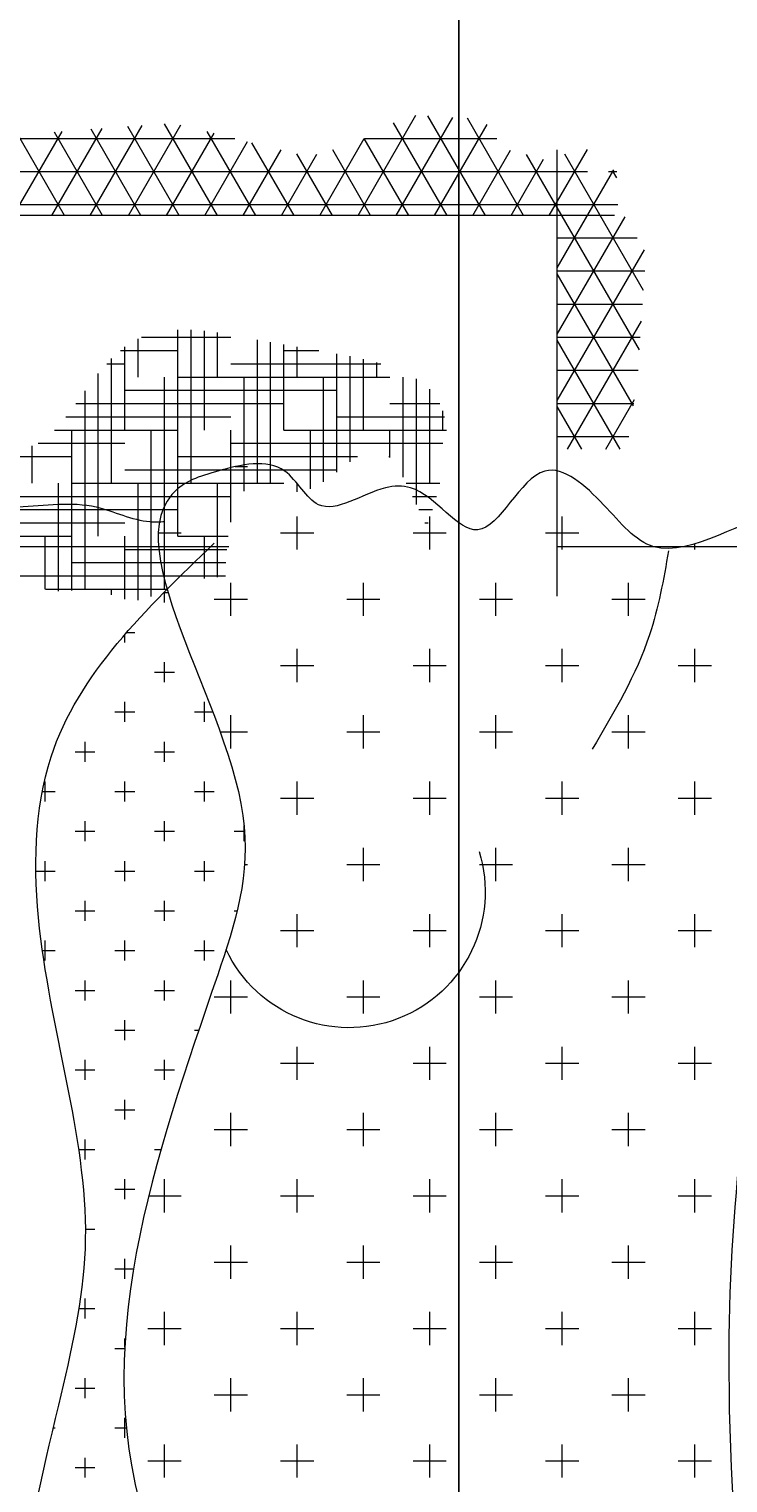
# Model space of a CAD drawing. Units: inches. Extents: x 3731 to 4318, y 1310 to 2388.
# Tile 19 of 57: x 4176 to 4203, y 1445 to 1502. Entities that reach past the tile are written whole.
import ezdxf

# ---------------------------------------------------------------- set-up
doc = ezdxf.new("R2010")
doc.units = ezdxf.units.IN
doc.layers.add('A-ANNO-DIMS', color=2, linetype='Continuous', lineweight=18)
doc.layers.add('A-FURN', color=8, linetype='Continuous', lineweight=13)
doc.styles.get("Standard").update_dxf_attribs({"font": 'arial.ttf'})
doc.dimstyles.get("Standard").update_dxf_attribs({"dimtxt": 0.18, "dimasz": 0.18, "dimexe": 0.18, "dimexo": 0.0625, "dimgap": 0.09, "dimtad": 0, "dimtih": 1, "dimtoh": 1, "dimdec": 4, "dimzin": 0, "dimdsep": 46, "dimtxsty": 'Standard', "dimcen": 0.09, "dimadec": 0, "dimazin": 0, "dimtfac": 1, "dimtdec": 4, "dimtofl": 0, "dimtmove": 0, "dimatfit": 3, "dimfxl": 1, "dimtolj": 1, "dimtzin": 0, "dimarcsym": 0})

# ---------------------------------------------------------------- blocks, each defined once
blk = doc.blocks.new('A$C200C7901')
for p, q in [((2, 1.6055), (2, 2.3334)), ((1.1379, 1.7195), (1.1379, 1.7508)), ((1.1222, 1.7352), (1.1535, 1.7352)), ((1.9972, 1.7352), (2.0027, 1.7352)), ((1.9972, 1.7352), (2.0027, 1.7352)), ((2, 1.6963), (2, 1.7248)), ((2, 1.6963), (2, 1.7248)), ((2.3121, 1.6596), (2.3121, 0.0201)), ((1.9533, 1.6055), (2.3741, 1.6055)), ((1.9533, 1.6055), (2.3741, 1.6055)), ((2, 0.2957), (2, 1.2957)), ((2.0224, 0.9977), (2.0224, 1.1977)), ((2.0224, 0.9977), (2.0224, 1.1977))]:
    blk.add_line(p, q)
at = {"linetype": 'ByBlock'}
for p, q in [((1.1379, 1.7195), (1.1379, 1.7508)), ((1.2629, 1.7195), (1.2629, 1.7508)), ((1.2629, 1.7195), (1.2629, 1.7508)), ((1.3879, 1.7195), (1.3879, 1.7508)), ((1.3879, 1.7195), (1.3879, 1.7508)), ((1.5129, 1.7195), (1.5129, 1.7508)), ((1.5129, 1.7195), (1.5129, 1.7508)), ((1.6379, 1.7195), (1.6379, 1.7508)), ((1.6379, 1.7195), (1.6379, 1.7508)), ((1.7629, 1.7195), (1.7629, 1.7508)), ((1.7629, 1.7195), (1.7629, 1.7508)), ((1.8879, 1.7195), (1.8879, 1.7508)), ((1.8879, 1.7195), (1.8879, 1.7508)), ((1.1222, 1.7352), (1.1535, 1.7352)), ((1.2472, 1.7352), (1.2785, 1.7352)), ((1.2472, 1.7352), (1.2785, 1.7352)), ((1.3722, 1.7352), (1.4035, 1.7352)), ((1.3722, 1.7352), (1.4035, 1.7352)), ((1.4972, 1.7352), (1.5285, 1.7352)), ((1.4972, 1.7352), (1.5285, 1.7352)), ((1.6222, 1.7352), (1.6535, 1.7352)), ((1.6222, 1.7352), (1.6535, 1.7352)), ((1.7472, 1.7352), (1.7785, 1.7352)), ((1.7472, 1.7352), (1.7785, 1.7352)), ((1.8722, 1.7352), (1.9035, 1.7352)), ((1.8722, 1.7352), (1.9035, 1.7352)), ((1.2004, 1.657), (1.2004, 1.6883)), ((1.2004, 1.657), (1.2004, 1.6883)), ((1.3254, 1.657), (1.3254, 1.6883)), ((1.3254, 1.657), (1.3254, 1.6883)), ((1.4504, 1.657), (1.4504, 1.6883)), ((1.4504, 1.657), (1.4504, 1.6883)), ((1.5754, 1.657), (1.5754, 1.6883)), ((1.5754, 1.657), (1.5754, 1.6883)), ((1.7004, 1.657), (1.7004, 1.6883)), ((1.7004, 1.657), (1.7004, 1.6883)), ((1.8254, 1.657), (1.8254, 1.6883)), ((1.8254, 1.657), (1.8254, 1.6883)), ((1.9504, 1.657), (1.9504, 1.6883)), ((1.9504, 1.657), (1.9504, 1.6883)), ((2.1377, 1.6055), (2.2798, 1.6876)), ((2.1377, 1.6055), (2.2798, 1.6876)), ((2.2414, 1.6868), (2.3699, 1.6126)), ((2.2414, 1.6868), (2.3699, 1.6126)), ((2.2599, 1.6055), (2.2599, 1.688)), ((2.2599, 1.6055), (2.2599, 1.688)), ((1.1847, 1.6727), (1.216, 1.6727)), ((1.1847, 1.6727), (1.216, 1.6727)), ((1.3097, 1.6727), (1.341, 1.6727)), ((1.3097, 1.6727), (1.341, 1.6727)), ((1.4347, 1.6727), (1.466, 1.6727)), ((1.4347, 1.6727), (1.466, 1.6727)), ((1.5597, 1.6727), (1.591, 1.6727)), ((1.5597, 1.6727), (1.591, 1.6727)), ((1.6847, 1.6727), (1.716, 1.6727)), ((1.6847, 1.6727), (1.716, 1.6727)), ((1.8097, 1.6727), (1.841, 1.6727)), ((1.8097, 1.6727), (1.841, 1.6727)), ((1.9347, 1.6727), (1.966, 1.6727)), ((1.9347, 1.6727), (1.966, 1.6727)), ((2.0919, 1.6152), (2.2125, 1.6848)), ((2.0919, 1.6152), (2.2125, 1.6848)), ((2.0919, 1.6513), (2.1386, 1.6782)), ((2.0919, 1.6513), (2.1386, 1.6782)), ((2.1037, 1.6055), (2.1037, 1.673)), ((2.1037, 1.6055), (2.1037, 1.673)), ((2.1327, 1.6773), (2.2571, 1.6055)), ((2.1327, 1.6773), (2.2571, 1.6055)), ((2.1349, 1.6055), (2.1349, 1.6777)), ((2.1349, 1.6055), (2.1349, 1.6777)), ((2.1662, 1.6055), (2.1662, 1.6817)), ((2.1662, 1.6055), (2.1662, 1.6817)), ((2.1854, 1.683), (2.3697, 1.5766)), ((2.1854, 1.683), (2.3697, 1.5766)), ((2.1974, 1.6055), (2.1974, 1.6838)), ((2.1974, 1.6055), (2.1974, 1.6838)), ((2.2287, 1.6055), (2.2287, 1.6859)), ((2.2287, 1.6055), (2.2287, 1.6859)), ((2.2912, 1.6055), (2.2912, 1.6809)), ((2.2912, 1.6055), (2.2912, 1.6809)), ((2.0919, 1.6649), (2.1946, 1.6055)), ((2.0919, 1.6649), (2.1946, 1.6055)), ((2.2002, 1.6055), (2.3109, 1.6694)), ((2.2002, 1.6055), (2.3109, 1.6694)), ((2.2627, 1.6055), (2.3551, 1.6589)), ((2.2627, 1.6055), (2.3551, 1.6589)), ((2.3224, 0.0468), (2.3224, 1.6627)), ((2.3224, 0.0468), (2.3224, 1.6627)), ((2.3476, 1.6616), (2.3547, 1.6575)), ((2.3476, 1.6616), (2.3547, 1.6575)), ((2.3537, 1.6539), (2.3537, 1.6616)), ((2.3537, 1.6539), (2.3537, 1.6616)), ((2.3121, 1.598), (2.3745, 1.634)), ((2.3121, 1.598), (2.3745, 1.634)), ((2.3537, 0.0056), (2.3537, 1.634)), ((2.3537, 0.0056), (2.3537, 1.634)), ((1.1379, 1.5945), (1.1379, 1.6258)), ((1.1379, 1.5945), (1.1379, 1.6258)), ((1.2629, 1.5945), (1.2629, 1.6258)), ((1.2629, 1.5945), (1.2629, 1.6258)), ((1.3879, 1.5945), (1.3879, 1.6258)), ((1.3879, 1.5945), (1.3879, 1.6258)), ((1.5129, 1.5945), (1.5129, 1.6258)), ((1.5129, 1.5945), (1.5129, 1.6258)), ((1.6379, 1.5945), (1.6379, 1.6258)), ((1.6379, 1.5945), (1.6379, 1.6258)), ((1.7629, 1.5945), (1.7629, 1.6258)), ((1.7629, 1.5945), (1.7629, 1.6258)), ((1.8879, 1.5945), (1.8879, 1.6258)), ((1.8879, 1.5945), (1.8879, 1.6258)), ((2.0129, 1.5945), (2.0129, 1.6258)), ((2.0129, 1.5945), (2.0129, 1.6258)), ((2.0919, 1.6288), (2.1321, 1.6055)), ((2.0919, 1.6288), (2.1321, 1.6055)), ((1.1222, 1.6102), (1.1535, 1.6102)), ((1.1222, 1.6102), (1.1535, 1.6102)), ((1.2472, 1.6102), (1.2785, 1.6102)), ((1.2472, 1.6102), (1.2785, 1.6102)), ((1.3722, 1.6102), (1.4035, 1.6102)), ((1.3722, 1.6102), (1.4035, 1.6102)), ((1.4972, 1.6102), (1.5285, 1.6102)), ((1.4972, 1.6102), (1.5285, 1.6102)), ((1.6222, 1.6102), (1.6535, 1.6102)), ((1.6222, 1.6102), (1.6535, 1.6102)), ((1.7472, 1.6102), (1.7785, 1.6102)), ((1.7472, 1.6102), (1.7785, 1.6102)), ((1.8722, 1.6102), (1.9035, 1.6102)), ((1.8722, 1.6102), (1.9035, 1.6102)), ((1.9972, 1.6102), (2.0285, 1.6102)), ((1.9972, 1.6102), (2.0285, 1.6102)), ((2.3121, 1.5619), (2.3654, 1.5926)), ((2.3121, 1.5619), (2.3654, 1.5926)), ((1.2004, 1.532), (1.2004, 1.5633)), ((1.2004, 1.532), (1.2004, 1.5633)), ((1.3254, 1.532), (1.3254, 1.5633)), ((1.3254, 1.532), (1.3254, 1.5633)), ((1.4504, 1.532), (1.4504, 1.5633)), ((1.4504, 1.532), (1.4504, 1.5633)), ((1.5754, 1.532), (1.5754, 1.5633)), ((1.5754, 1.532), (1.5754, 1.5633)), ((1.7004, 1.532), (1.7004, 1.5633)), ((1.7004, 1.532), (1.7004, 1.5633)), ((1.8254, 1.532), (1.8254, 1.5633)), ((1.8254, 1.532), (1.8254, 1.5633)), ((1.9504, 1.532), (1.9504, 1.5633)), ((1.9504, 1.532), (1.9504, 1.5633)), ((2.3121, 1.5738), (2.404, 1.5208)), ((2.3121, 1.5738), (2.404, 1.5208)), ((2.3121, 1.5258), (2.3739, 1.5615)), ((2.3121, 1.5258), (2.3739, 1.5615)), ((1.1847, 1.5477), (1.216, 1.5477)), ((1.1847, 1.5477), (1.216, 1.5477)), ((1.3097, 1.5477), (1.341, 1.5477)), ((1.3097, 1.5477), (1.341, 1.5477)), ((1.4347, 1.5477), (1.466, 1.5477)), ((1.4347, 1.5477), (1.466, 1.5477)), ((1.5597, 1.5477), (1.591, 1.5477)), ((1.5597, 1.5477), (1.591, 1.5477)), ((1.6847, 1.5477), (1.716, 1.5477)), ((1.6847, 1.5477), (1.716, 1.5477)), ((1.8097, 1.5477), (1.841, 1.5477)), ((1.8097, 1.5477), (1.841, 1.5477)), ((1.9347, 1.5477), (1.966, 1.5477)), ((1.9347, 1.5477), (1.966, 1.5477)), ((2.3121, 1.4897), (2.3979, 1.5393)), ((2.3121, 1.4897), (2.3979, 1.5393)), ((2.3121, 1.5377), (2.406, 1.4835)), ((2.3121, 1.5377), (2.406, 1.4835)), ((2.3849, 1.4236), (2.3849, 1.5486)), ((2.3849, 1.4236), (2.3849, 1.5486)), ((1.1379, 1.4695), (1.1379, 1.5008)), ((1.1379, 1.4695), (1.1379, 1.5008)), ((1.2629, 1.4695), (1.2629, 1.5008)), ((1.2629, 1.4695), (1.2629, 1.5008)), ((1.3879, 1.4695), (1.3879, 1.5008)), ((1.3879, 1.4695), (1.3879, 1.5008)), ((1.5129, 1.4695), (1.5129, 1.5008)), ((1.5129, 1.4695), (1.5129, 1.5008)), ((1.6379, 1.4695), (1.6379, 1.5008)), ((1.6379, 1.4695), (1.6379, 1.5008)), ((1.7629, 1.4695), (1.7629, 1.5008)), ((1.7629, 1.4695), (1.7629, 1.5008)), ((1.8879, 1.4695), (1.8879, 1.5008)), ((1.8879, 1.4695), (1.8879, 1.5008)), ((2.0129, 1.4695), (2.0129, 1.5008)), ((2.0129, 1.4695), (2.0129, 1.5008)), ((2.0599, 1.4631), (2.0599, 1.4948)), ((2.0599, 1.4631), (2.0599, 1.4948)), ((2.0974, 1.2977), (2.0974, 1.4977)), ((2.0974, 1.2977), (2.0974, 1.4977)), ((2.1099, 1.3477), (2.1099, 1.5009)), ((2.1099, 1.3477), (2.1099, 1.5009)), ((2.1099, 1.4977), (2.1279, 1.4977)), ((2.1099, 1.4977), (2.1279, 1.4977)), ((2.1224, 1.3977), (2.1224, 1.4992)), ((2.1224, 1.3977), (2.1224, 1.4992)), ((2.1349, 1.4477), (2.1349, 1.4949)), ((2.1349, 1.4477), (2.1349, 1.4949)), ((2.3121, 1.4537), (2.4047, 1.5071)), ((2.3121, 1.4537), (2.4047, 1.5071)), ((2.3121, 1.5016), (2.3997, 1.4511)), ((2.3121, 1.5016), (2.3997, 1.4511)), ((1.1222, 1.4852), (1.1535, 1.4852)), ((1.1222, 1.4852), (1.1535, 1.4852)), ((1.2472, 1.4852), (1.2785, 1.4852)), ((1.2472, 1.4852), (1.2785, 1.4852)), ((1.3722, 1.4852), (1.4035, 1.4852)), ((1.3722, 1.4852), (1.4035, 1.4852)), ((1.4972, 1.4852), (1.5285, 1.4852)), ((1.4972, 1.4852), (1.5285, 1.4852)), ((1.6222, 1.4852), (1.6535, 1.4852)), ((1.6222, 1.4852), (1.6535, 1.4852)), ((1.7472, 1.4852), (1.7785, 1.4852)), ((1.7472, 1.4852), (1.7785, 1.4852)), ((1.8722, 1.4852), (1.9035, 1.4852)), ((1.8722, 1.4852), (1.9035, 1.4852)), ((1.9972, 1.4852), (2.0285, 1.4852)), ((1.9972, 1.4852), (2.0285, 1.4852)), ((2.0224, 1.4805), (2.0224, 1.4839)), ((2.0224, 1.4805), (2.0224, 1.4839)), ((2.0349, 1.4748), (2.0349, 1.4879)), ((2.0349, 1.4748), (2.0349, 1.4879)), ((2.0474, 1.4691), (2.0474, 1.4915)), ((2.0474, 1.4691), (2.0474, 1.4915)), ((2.0599, 1.4852), (2.1484, 1.4852)), ((2.0599, 1.4852), (2.1484, 1.4852)), ((2.0397, 1.4727), (2.1581, 1.4727)), ((2.0397, 1.4727), (2.1581, 1.4727)), ((2.3121, 1.4176), (2.4067, 1.4721)), ((2.3121, 1.4176), (2.4067, 1.4721)), ((2.0656, 1.4602), (2.1599, 1.4602)), ((2.0656, 1.4602), (2.1599, 1.4602)), ((2.3121, 1.4655), (2.3849, 1.4235)), ((2.3121, 1.4655), (2.3849, 1.4235)), ((2.084, 1.4477), (2.1099, 1.4477)), ((2.084, 1.4477), (2.1099, 1.4477)), ((2.0849, 1.4468), (2.0849, 1.4477)), ((2.0849, 1.4468), (2.0849, 1.4477)), ((2.1599, 1.2477), (2.1599, 1.4477)), ((2.1599, 1.2477), (2.1599, 1.4477)), ((1.2004, 1.407), (1.2004, 1.4383)), ((1.2004, 1.407), (1.2004, 1.4383)), ((1.3254, 1.407), (1.3254, 1.4383)), ((1.3254, 1.407), (1.3254, 1.4383)), ((1.4504, 1.407), (1.4504, 1.4383)), ((1.4504, 1.407), (1.4504, 1.4383)), ((1.5754, 1.407), (1.5754, 1.4383)), ((1.5754, 1.407), (1.5754, 1.4383)), ((1.7004, 1.407), (1.7004, 1.4383)), ((1.7004, 1.407), (1.7004, 1.4383)), ((1.8254, 1.407), (1.8254, 1.4383)), ((1.8254, 1.407), (1.8254, 1.4383)), ((1.9504, 1.407), (1.9504, 1.4383)), ((1.9504, 1.407), (1.9504, 1.4383)), ((2.1599, 1.4352), (2.1735, 1.4352)), ((2.1599, 1.4352), (2.1735, 1.4352)), ((2.1724, 1.2977), (2.1724, 1.439)), ((2.1724, 1.2977), (2.1724, 1.439)), ((2.3121, 1.4294), (2.3741, 1.3937)), ((2.3121, 1.4294), (2.3741, 1.3937)), ((1.1847, 1.4227), (1.216, 1.4227)), ((1.1847, 1.4227), (1.216, 1.4227)), ((1.3097, 1.4227), (1.341, 1.4227)), ((1.3097, 1.4227), (1.341, 1.4227)), ((1.4347, 1.4227), (1.466, 1.4227)), ((1.4347, 1.4227), (1.466, 1.4227)), ((1.5597, 1.4227), (1.591, 1.4227)), ((1.5597, 1.4227), (1.591, 1.4227)), ((1.6847, 1.4227), (1.716, 1.4227)), ((1.6847, 1.4227), (1.716, 1.4227)), ((1.8097, 1.4227), (1.841, 1.4227)), ((1.8097, 1.4227), (1.841, 1.4227)), ((1.9347, 1.4227), (1.966, 1.4227)), ((1.9347, 1.4227), (1.966, 1.4227)), ((2.0849, 1.2477), (2.0849, 1.4171)), ((2.0849, 1.2477), (2.0849, 1.4171)), ((2.1099, 1.4227), (2.1767, 1.4227)), ((2.1099, 1.4227), (2.1767, 1.4227)), ((2.3121, 1.3815), (2.3848, 1.4235)), ((2.3121, 1.3815), (2.3848, 1.4235)), ((2.08, 1.4102), (2.1795, 1.4102)), ((2.08, 1.4102), (2.1795, 1.4102)), ((2.0612, 1.3852), (2.1599, 1.3852)), ((2.0612, 1.3852), (2.1599, 1.3852)), ((2.0703, 1.3977), (2.1819, 1.3977)), ((2.0703, 1.3977), (2.1819, 1.3977)), ((2.0724, 1.1977), (2.0724, 1.3977)), ((2.0724, 1.1977), (2.0724, 1.3977)), ((2.1474, 1.1977), (2.1474, 1.3977)), ((2.1474, 1.1977), (2.1474, 1.3977)), ((2.3121, 1.3934), (2.3703, 1.3598)), ((2.3121, 1.3934), (2.3703, 1.3598)), ((1.1379, 1.3445), (1.1379, 1.3758)), ((1.1379, 1.3445), (1.1379, 1.3758)), ((1.2629, 1.3445), (1.2629, 1.3758)), ((1.2629, 1.3445), (1.2629, 1.3758)), ((1.3879, 1.3445), (1.3879, 1.3758)), ((1.3879, 1.3445), (1.3879, 1.3758)), ((1.5129, 1.3445), (1.5129, 1.3758)), ((1.5129, 1.3445), (1.5129, 1.3758)), ((1.6379, 1.3445), (1.6379, 1.3758)), ((1.6379, 1.3445), (1.6379, 1.3758)), ((1.7629, 1.3445), (1.7629, 1.3758)), ((1.7629, 1.3445), (1.7629, 1.3758)), ((1.8879, 1.3445), (1.8879, 1.3758)), ((1.8879, 1.3445), (1.8879, 1.3758)), ((2.0129, 1.3445), (2.0129, 1.3758)), ((2.0129, 1.3445), (2.0129, 1.3758)), ((2.0545, 1.3727), (2.1099, 1.3727)), ((2.0545, 1.3727), (2.1099, 1.3727)), ((2.1849, 1.3477), (2.1849, 1.3808)), ((2.1849, 1.3477), (2.1849, 1.3808)), ((2.3121, 1.3454), (2.37, 1.3788)), ((2.3121, 1.3454), (2.37, 1.3788)), ((1.1222, 1.3602), (1.1535, 1.3602)), ((1.1222, 1.3602), (1.1535, 1.3602)), ((1.2472, 1.3602), (1.2785, 1.3602)), ((1.2472, 1.3602), (1.2785, 1.3602)), ((1.3722, 1.3602), (1.4035, 1.3602)), ((1.3722, 1.3602), (1.4035, 1.3602)), ((1.4972, 1.3602), (1.5285, 1.3602)), ((1.4972, 1.3602), (1.5285, 1.3602)), ((1.6222, 1.3602), (1.6535, 1.3602)), ((1.6222, 1.3602), (1.6535, 1.3602)), ((1.7472, 1.3602), (1.7785, 1.3602)), ((1.7472, 1.3602), (1.7785, 1.3602)), ((1.8722, 1.3602), (1.9035, 1.3602)), ((1.8722, 1.3602), (1.9035, 1.3602)), ((1.9972, 1.3602), (2.0285, 1.3602)), ((1.9972, 1.3602), (2.0285, 1.3602)), ((2.0515, 1.3602), (2.0599, 1.3602)), ((2.0515, 1.3602), (2.0599, 1.3602)), ((2.1599, 1.3602), (2.1883, 1.3602)), ((2.1599, 1.3602), (2.1883, 1.3602)), ((2.3121, 1.3573), (2.3808, 1.3176)), ((2.3121, 1.3573), (2.3808, 1.3176)), ((2.0599, 1.1477), (2.0599, 1.3477)), ((2.0599, 1.1477), (2.0599, 1.3477)), ((2.1099, 1.3477), (2.1904, 1.3477)), ((2.1099, 1.3477), (2.1904, 1.3477)), ((2.1349, 1.1515), (2.1349, 1.3477)), ((2.1349, 1.1515), (2.1349, 1.3477)), ((2.3121, 1.3093), (2.374, 1.345)), ((2.3121, 1.3093), (2.374, 1.345)), ((2.0599, 1.3352), (2.1926, 1.3352)), ((2.0599, 1.3352), (2.1926, 1.3352)), ((2.0594, 1.3227), (2.195, 1.3227)), ((2.0594, 1.3227), (2.195, 1.3227)), ((2.3121, 1.3212), (2.3914, 1.2754)), ((2.3121, 1.3212), (2.3914, 1.2754)), ((1.2004, 1.282), (1.2004, 1.3133)), ((1.2004, 1.282), (1.2004, 1.3133)), ((1.3254, 1.282), (1.3254, 1.3133)), ((1.3254, 1.282), (1.3254, 1.3133)), ((1.4504, 1.282), (1.4504, 1.3133)), ((1.4504, 1.282), (1.4504, 1.3133)), ((1.5754, 1.282), (1.5754, 1.3133)), ((1.5754, 1.282), (1.5754, 1.3133)), ((1.6566, 1.3008), (1.6566, 1.3036)), ((1.6566, 1.3008), (1.6566, 1.3036)), ((1.7004, 1.3106), (1.7004, 1.3133)), ((1.7004, 1.3106), (1.7004, 1.3133)), ((1.7222, 1.3102), (1.7369, 1.3102)), ((1.7222, 1.3102), (1.7369, 1.3102)), ((1.7316, 1.3008), (1.7316, 1.3106)), ((1.7316, 1.3008), (1.7316, 1.3106)), ((1.8254, 1.2876), (1.8254, 1.3133)), ((1.8254, 1.2876), (1.8254, 1.3133)), ((1.9504, 1.282), (1.9504, 1.3133)), ((1.9504, 1.282), (1.9504, 1.3133)), ((2.0524, 1.3102), (2.1599, 1.3102)), ((2.0524, 1.3102), (2.1599, 1.3102)), ((2.0754, 1.3017), (2.0754, 1.3133)), ((2.0754, 1.3017), (2.0754, 1.3133)), ((2.3121, 1.2732), (2.3819, 1.3135)), ((2.3121, 1.2732), (2.3819, 1.3135)), ((1.1847, 1.2977), (1.216, 1.2977)), ((1.1847, 1.2977), (1.216, 1.2977)), ((1.3097, 1.2977), (1.341, 1.2977)), ((1.3097, 1.2977), (1.341, 1.2977)), ((1.4347, 1.2977), (1.466, 1.2977)), ((1.4347, 1.2977), (1.466, 1.2977)), ((1.5597, 1.2977), (1.591, 1.2977)), ((1.5597, 1.2977), (1.591, 1.2977)), ((1.8097, 1.2977), (1.841, 1.2977)), ((1.8097, 1.2977), (1.841, 1.2977)), ((1.9347, 1.2977), (1.966, 1.2977)), ((1.9347, 1.2977), (1.966, 1.2977)), ((1.9724, 1.0977), (1.9724, 1.2927)), ((1.9724, 1.0977), (1.9724, 1.2927)), ((1.9849, 1.1477), (1.9849, 1.293)), ((1.9849, 1.1477), (1.9849, 1.293)), ((1.9974, 1.1977), (1.9974, 1.2939)), ((1.9974, 1.1977), (1.9974, 1.2939)), ((2.0099, 1.2477), (2.0099, 1.2953)), ((2.0099, 1.2477), (2.0099, 1.2953)), ((2.023, 1.2977), (2.1099, 1.2977)), ((2.023, 1.2977), (2.1099, 1.2977)), ((2.0474, 1.0977), (2.0474, 1.2977)), ((2.0474, 1.0977), (2.0474, 1.2977)), ((2.0597, 1.2977), (2.0744, 1.2977)), ((2.0597, 1.2977), (2.0744, 1.2977)), ((2.1224, 1.1421), (2.1224, 1.2977)), ((2.1224, 1.1421), (2.1224, 1.2977)), ((2.1974, 1.2135), (2.1974, 1.2977)), ((2.1974, 1.2135), (2.1974, 1.2977)), ((2.3849, 1.0607), (2.3849, 1.3013)), ((2.3849, 1.0607), (2.3849, 1.3013)), ((1.6191, 1.2633), (1.6191, 1.282)), ((1.6191, 1.2633), (1.6191, 1.282)), ((1.6941, 1.2633), (1.6941, 1.282)), ((1.6941, 1.2633), (1.6941, 1.282)), ((1.7691, 1.2633), (1.7691, 1.282)), ((1.7691, 1.2633), (1.7691, 1.282)), ((1.8441, 1.2633), (1.8441, 1.2806)), ((1.8441, 1.2633), (1.8441, 1.2806)), ((1.9711, 1.2852), (2.0599, 1.2852)), ((1.9711, 1.2852), (2.0599, 1.2852)), ((2.1599, 1.2852), (2.2018, 1.2852)), ((2.1599, 1.2852), (2.2018, 1.2852)), ((2.3121, 1.2851), (2.3985, 1.2352)), ((2.3121, 1.2851), (2.3985, 1.2352)), ((2.3121, 1.2371), (2.3898, 1.282)), ((2.3121, 1.2371), (2.3898, 1.282)), ((1.5441, 1.2633), (1.5441, 1.2675)), ((1.5441, 1.2633), (1.5441, 1.2675)), ((1.6097, 1.2727), (1.6285, 1.2727)), ((1.6097, 1.2727), (1.6285, 1.2727)), ((1.6847, 1.2727), (1.7035, 1.2727)), ((1.6847, 1.2727), (1.7035, 1.2727)), ((1.7597, 1.2727), (1.7785, 1.2727)), ((1.7597, 1.2727), (1.7785, 1.2727)), ((1.8347, 1.2727), (1.8535, 1.2727)), ((1.8347, 1.2727), (1.8535, 1.2727)), ((1.97, 1.2727), (2.0099, 1.2727)), ((1.97, 1.2727), (2.0099, 1.2727)), ((2.1099, 1.2727), (2.2034, 1.2727)), ((2.1099, 1.2727), (2.2034, 1.2727)), ((1.1379, 1.2195), (1.1379, 1.2508)), ((1.1379, 1.2195), (1.1379, 1.2508)), ((1.2629, 1.2195), (1.2629, 1.2508)), ((1.2629, 1.2195), (1.2629, 1.2508)), ((1.3879, 1.2202), (1.3879, 1.2508)), ((1.3879, 1.2202), (1.3879, 1.2508)), ((2.0099, 1.2477), (2.2045, 1.2477)), ((2.0099, 1.2477), (2.2045, 1.2477)), ((2.0129, 1.2293), (2.0129, 1.2508)), ((2.0129, 1.2293), (2.0129, 1.2508)), ((2.0349, 1.0477), (2.0349, 1.2477)), ((2.0349, 1.0477), (2.0349, 1.2477)), ((2.0599, 1.2602), (2.2044, 1.2602)), ((2.0599, 1.2602), (2.2044, 1.2602)), ((2.1099, 1.1315), (2.1099, 1.2477)), ((2.1099, 1.1315), (2.1099, 1.2477)), ((2.1849, 1.1935), (2.1849, 1.2477)), ((2.1849, 1.1935), (2.1849, 1.2477)), ((2.3121, 1.2011), (2.3976, 1.2504)), ((2.3121, 1.2011), (2.3976, 1.2504)), ((2.3121, 1.249), (2.396, 1.2006)), ((2.3121, 1.249), (2.396, 1.2006)), ((1.1222, 1.2352), (1.1535, 1.2352)), ((1.1222, 1.2352), (1.1535, 1.2352)), ((1.2472, 1.2352), (1.2785, 1.2352)), ((1.2472, 1.2352), (1.2785, 1.2352)), ((1.3722, 1.2352), (1.4035, 1.2352)), ((1.3722, 1.2352), (1.4035, 1.2352)), ((1.4972, 1.2352), (1.516, 1.2352)), ((1.4972, 1.2352), (1.516, 1.2352)), ((1.5066, 1.2258), (1.5066, 1.2445)), ((1.5066, 1.2258), (1.5066, 1.2445)), ((1.5722, 1.2352), (1.591, 1.2352)), ((1.5722, 1.2352), (1.591, 1.2352)), ((1.5816, 1.2258), (1.5816, 1.2445)), ((1.5816, 1.2258), (1.5816, 1.2445)), ((1.6472, 1.2352), (1.666, 1.2352)), ((1.6472, 1.2352), (1.666, 1.2352)), ((1.6566, 1.2258), (1.6566, 1.2445)), ((1.6566, 1.2258), (1.6566, 1.2445)), ((1.7222, 1.2352), (1.741, 1.2352)), ((1.7222, 1.2352), (1.741, 1.2352)), ((1.7316, 1.2258), (1.7316, 1.2445)), ((1.7316, 1.2258), (1.7316, 1.2445)), ((1.7972, 1.2352), (1.816, 1.2352)), ((1.7972, 1.2352), (1.816, 1.2352)), ((1.8066, 1.2258), (1.8066, 1.2445)), ((1.8066, 1.2258), (1.8066, 1.2445)), ((1.8722, 1.2352), (1.891, 1.2352)), ((1.8722, 1.2352), (1.891, 1.2352)), ((1.8816, 1.2258), (1.8816, 1.2445)), ((1.8816, 1.2258), (1.8816, 1.2445)), ((1.9472, 1.2352), (1.9574, 1.2352)), ((1.9472, 1.2352), (1.9574, 1.2352)), ((1.9566, 1.2344), (1.9566, 1.2385)), ((1.9566, 1.2344), (1.9566, 1.2385)), ((1.9599, 1.1228), (1.9599, 1.2373)), ((1.9599, 1.1228), (1.9599, 1.2373)), ((1.9599, 1.2352), (2.1599, 1.2352)), ((1.9599, 1.2352), (2.1599, 1.2352)), ((2, 1.2352), (2.0285, 1.2352)), ((2, 1.2352), (2.0285, 1.2352)), ((1.4316, 1.2258), (1.4316, 1.2318)), ((1.4316, 1.2258), (1.4316, 1.2318)), ((1.953, 1.2227), (2.1099, 1.2227)), ((1.953, 1.2227), (2.1099, 1.2227)), ((1.3941, 1.1883), (1.3941, 1.207)), ((1.3941, 1.1883), (1.3941, 1.207)), ((1.4691, 1.1883), (1.4691, 1.207)), ((1.4691, 1.1883), (1.4691, 1.207)), ((1.5441, 1.1883), (1.5441, 1.207)), ((1.5441, 1.1883), (1.5441, 1.207)), ((1.6191, 1.1883), (1.6191, 1.207)), ((1.6191, 1.1883), (1.6191, 1.207)), ((1.6941, 1.1883), (1.6941, 1.207)), ((1.6941, 1.1883), (1.6941, 1.207)), ((1.7691, 1.1883), (1.7691, 1.207)), ((1.7691, 1.1883), (1.7691, 1.207)), ((1.8441, 1.1883), (1.8441, 1.207)), ((1.8441, 1.1883), (1.8441, 1.207)), ((1.9191, 1.1995), (1.9191, 1.207)), ((1.9191, 1.1995), (1.9191, 1.207)), ((1.9495, 1.2102), (2.0599, 1.2102)), ((1.9495, 1.2102), (2.0599, 1.2102)), ((2.1599, 1.2102), (2.1959, 1.2102)), ((2.1599, 1.2102), (2.1959, 1.2102)), ((2.3121, 1.165), (2.397, 1.214)), ((2.3121, 1.165), (2.397, 1.214)), ((2.3121, 1.2129), (2.3935, 1.166)), ((2.3121, 1.2129), (2.3935, 1.166)), ((1.1597, 1.1977), (1.1785, 1.1977)), ((1.1597, 1.1977), (1.1785, 1.1977)), ((1.1691, 1.1883), (1.1691, 1.1991)), ((1.1691, 1.1883), (1.1691, 1.1991)), ((1.2441, 1.1883), (1.2441, 1.1976)), ((1.2441, 1.1883), (1.2441, 1.1976)), ((1.2452, 1.1977), (1.2535, 1.1977)), ((1.2452, 1.1977), (1.2535, 1.1977)), ((1.3097, 1.1977), (1.3285, 1.1977)), ((1.3097, 1.1977), (1.3285, 1.1977)), ((1.3191, 1.1883), (1.3191, 1.2059)), ((1.3191, 1.1883), (1.3191, 1.2059)), ((1.3847, 1.1977), (1.4035, 1.1977)), ((1.3847, 1.1977), (1.4035, 1.1977)), ((1.4597, 1.1977), (1.4785, 1.1977)), ((1.4597, 1.1977), (1.4785, 1.1977)), ((1.5347, 1.1977), (1.5535, 1.1977)), ((1.5347, 1.1977), (1.5535, 1.1977)), ((1.6097, 1.1977), (1.6285, 1.1977)), ((1.6097, 1.1977), (1.6285, 1.1977)), ((1.6847, 1.1977), (1.7035, 1.1977)), ((1.6847, 1.1977), (1.7035, 1.1977)), ((1.7597, 1.1977), (1.7785, 1.1977)), ((1.7597, 1.1977), (1.7785, 1.1977)), ((1.8347, 1.1977), (1.8535, 1.1977)), ((1.8347, 1.1977), (1.8535, 1.1977)), ((1.9097, 1.1977), (1.917, 1.1977)), ((1.9097, 1.1977), (1.917, 1.1977)), ((1.9506, 1.1977), (2.0099, 1.1977)), ((1.9506, 1.1977), (2.0099, 1.1977)), ((2.0974, 1.1161), (2.0974, 1.1977)), ((2.0974, 1.1161), (2.0974, 1.1977)), ((2.1099, 1.1977), (2.1882, 1.1977)), ((2.1099, 1.1977), (2.1882, 1.1977)), ((2.1724, 1.1807), (2.1724, 1.1977)), ((2.1724, 1.1807), (2.1724, 1.1977)), ((1.9545, 1.1852), (1.9599, 1.1852)), ((1.9545, 1.1852), (1.9599, 1.1852)), ((2.0599, 1.1852), (2.1772, 1.1852)), ((2.0599, 1.1852), (2.1772, 1.1852)), ((1.1316, 1.1508), (1.1316, 1.1695)), ((1.1316, 1.1508), (1.1316, 1.1695)), ((1.2066, 1.1508), (1.2066, 1.1695)), ((1.2066, 1.1508), (1.2066, 1.1695)), ((1.2816, 1.1547), (1.2816, 1.1695)), ((1.2816, 1.1547), (1.2816, 1.1695)), ((1.3566, 1.1608), (1.3566, 1.1695)), ((1.3566, 1.1608), (1.3566, 1.1695)), ((1.4316, 1.1544), (1.4316, 1.1695)), ((1.4316, 1.1544), (1.4316, 1.1695)), ((1.5066, 1.1508), (1.5066, 1.1695)), ((1.5066, 1.1508), (1.5066, 1.1695)), ((1.5816, 1.1508), (1.5816, 1.1695)), ((1.5816, 1.1508), (1.5816, 1.1695)), ((1.6566, 1.1508), (1.6566, 1.1695)), ((1.6566, 1.1508), (1.6566, 1.1695)), ((1.7316, 1.1508), (1.7316, 1.1695)), ((1.7316, 1.1508), (1.7316, 1.1695)), ((1.8066, 1.1508), (1.8066, 1.1695)), ((1.8066, 1.1508), (1.8066, 1.1695)), ((2.0099, 1.1727), (2.1631, 1.1727)), ((2.0099, 1.1727), (2.1631, 1.1727)), ((2.3121, 1.1768), (2.3909, 1.1314)), ((2.3121, 1.1768), (2.3909, 1.1314)), ((2.3121, 1.1289), (2.3942, 1.1763)), ((2.3121, 1.1289), (2.3942, 1.1763)), ((1.1222, 1.1602), (1.141, 1.1602)), ((1.1222, 1.1602), (1.141, 1.1602)), ((1.1972, 1.1602), (1.216, 1.1602)), ((1.1972, 1.1602), (1.216, 1.1602)), ((1.2722, 1.1602), (1.291, 1.1602)), ((1.2722, 1.1602), (1.291, 1.1602)), ((1.4222, 1.1602), (1.441, 1.1602)), ((1.4222, 1.1602), (1.441, 1.1602)), ((1.4972, 1.1602), (1.516, 1.1602)), ((1.4972, 1.1602), (1.516, 1.1602)), ((1.5722, 1.1602), (1.591, 1.1602)), ((1.5722, 1.1602), (1.591, 1.1602)), ((1.6472, 1.1602), (1.666, 1.1602)), ((1.6472, 1.1602), (1.666, 1.1602)), ((1.7222, 1.1602), (1.741, 1.1602)), ((1.7222, 1.1602), (1.741, 1.1602)), ((1.7972, 1.1602), (1.816, 1.1602)), ((1.7972, 1.1602), (1.816, 1.1602)), ((1.9599, 1.1602), (2.1468, 1.1602)), ((1.9599, 1.1602), (2.1468, 1.1602)), ((1.9585, 1.1477), (2.1099, 1.1477)), ((1.9585, 1.1477), (2.1099, 1.1477)), ((2.0099, 0.9477), (2.0099, 1.1477)), ((2.0099, 0.9477), (2.0099, 1.1477)), ((2.0849, 0.9477), (2.0849, 1.1477)), ((2.0849, 0.9477), (2.0849, 1.1477)), ((2.3121, 1.1408), (2.3884, 1.0967)), ((2.3121, 1.1408), (2.3884, 1.0967)), ((2.3121, 1.0928), (2.3915, 1.1386)), ((2.3121, 1.0928), (2.3915, 1.1386)), ((1.1691, 1.1303), (1.1691, 1.132)), ((1.1691, 1.1303), (1.1691, 1.132)), ((1.6191, 1.1201), (1.6191, 1.132)), ((1.6191, 1.1201), (1.6191, 1.132)), ((1.6941, 1.1139), (1.6941, 1.132)), ((1.6941, 1.1139), (1.6941, 1.132)), ((1.7691, 1.1198), (1.7691, 1.132)), ((1.7691, 1.1198), (1.7691, 1.132)), ((1.9581, 1.1352), (2.0599, 1.1352)), ((1.9581, 1.1352), (2.0599, 1.1352)), ((1.6097, 1.1227), (1.6285, 1.1227)), ((1.6097, 1.1227), (1.6285, 1.1227)), ((1.6847, 1.1227), (1.7035, 1.1227)), ((1.6847, 1.1227), (1.7035, 1.1227)), ((1.7597, 1.1227), (1.7785, 1.1227)), ((1.7597, 1.1227), (1.7785, 1.1227)), ((1.9599, 1.1227), (2.0099, 1.1227)), ((1.9599, 1.1227), (2.0099, 1.1227)), ((2.0599, 1.1102), (2.0951, 1.1102)), ((2.0599, 1.1102), (2.0951, 1.1102))]:
    blk.add_line(p, q, dxfattribs=at)
blk.add_arc((1.6746, 1.4093), 0.1282, 72.7909, 244.8695, dxfattribs=at)
blk.add_arc((1.6746, 1.4093), 0.1282, 72.7909, 244.8695, dxfattribs=at)
for points, knots in [([(0.4485, 1.7835), (0.4321, 1.7496), (0.4062, 1.6964), (0.49, 1.6713), (0.4719, 1.5969), (0.4123, 1.592), (0.4233, 1.5337), (0.4954, 1.5086), (0.4012, 1.4738), (0.3253, 1.4306), (0.4113, 1.3764), (0.3688, 1.3065), (0.5579, 1.2663), (0.741, 1.4533), (1.1127, 1.1109), (1.4811, 1.2478), (1.7885, 1.3492), (2.0357, 1.1637), (2.0748, 1.2974), (2.0876, 1.349), (2.0192, 1.3805), (2.0564, 1.4298), (2.0588, 1.4846), (1.9759, 1.5349), (2.1004, 1.5845), (2.0397, 1.6519), (1.971, 1.7053), (2.1104, 1.8981), (1.5946, 1.7967), (1.2448, 1.7472), (0.8129, 1.7935), (0.4953, 1.8548), (0.4582, 1.7983), (0.4485, 1.7835)], [0, 0, 0, 0, 88.420092, 139.08588, 204.302936, 239.695496, 287.801042, 327.365471, 412.960499, 463.626286, 552.059846, 584.668336, 662.614915, 940.993281, 1309.926334, 1844.022653, 1996.276242, 2316.43048, 2341.441004, 2404.707416, 2449.463774, 2514.680778, 2538.40571, 2613.031547, 2697.13096, 2760.903931, 2822.692699, 2945.47, 3215.060018, 3725.584917, 4361.974444, 4504.671998, 4555.32777, 4555.32777, 4555.32777, 4555.32777]), ([(0.4856, 1.3429), (0.5504, 1.3182), (0.6715, 1.2721), (0.8374, 1.0498), (1.1164, 1.1183), (1.3878, 1.1816), (1.5888, 1.1102), (1.8403, 1.1127), (1.9415, 1.2178), (2.0032, 1.2819)], [0, 0, 0, 0, 205.411753, 383.654933, 772.067458, 921.644661, 1226.793228, 1388.983508, 1642.292305, 1642.292305, 1642.292305, 1642.292305])]:
    blk.add_open_spline(points, degree=3, knots=knots)
for points, knots in [([(1.996, 1.7104), (1.9692, 1.7057), (1.9025, 1.6938), (1.844, 1.6592), (1.809, 1.6385)], [0, 0, 0, 0, 81.132613, 201.738644, 201.738644, 201.738644, 201.738644]), ([(1.996, 1.7104), (1.9692, 1.7057), (1.9025, 1.6938), (1.844, 1.6592), (1.809, 1.6385)], [0, 0, 0, 0, 81.132613, 201.738644, 201.738644, 201.738644, 201.738644]), ([(0.473, 1.2954), (0.4739, 1.2781), (0.4755, 1.2477), (0.5032, 1.2084), (0.4801, 1.1701), (0.4928, 1.1255), (0.4674, 1.0912), (0.4579, 1.0351), (0.501, 0.9724), (0.4311, 0.8832), (0.4902, 0.8637), (0.4843, 0.8288), (0.4774, 0.7906), (0.4625, 0.7457), (0.459, 0.6999), (0.4816, 0.6664), (0.4748, 0.625), (0.4791, 0.5889), (0.4533, 0.5528), (0.4738, 0.5004), (0.4658, 0.4502), (0.4696, 0.3946), (0.4189, 0.3935), (0.4493, 0.3684), (0.4694, 0.3857), (0.4922, 0.3576), (0.5297, 0.3262), (0.5917, 0.3353), (0.6454, 0.3754), (0.7083, 0.3741), (0.7643, 0.3328), (0.826, 0.346), (0.925, 0.3388), (1.0353, 0.3593), (1.1561, 0.3744), (1.2477, 0.3154), (1.3302, 0.3474), (1.4086, 0.3512), (1.5217, 0.3878), (1.6362, 0.3176), (1.7682, 0.3285), (1.8402, 0.3019), (1.9071, 0.3529), (1.9647, 0.3412), (2.0795, 0.2948), (2.0472, 0.3498), (2.0343, 0.3772), (2.0435, 0.43), (2.0109, 0.5782), (2.0746, 0.4643), (2.0805, 0.584), (2.0084, 0.5979), (2.0343, 0.6846), (2.0344, 0.746), (2.0293, 0.8096), (2.0489, 0.8545), (2.0652, 0.9218), (1.9842, 0.9297), (2.0007, 1.0162), (2.0367, 1.0585), (2.0367, 1.1102), (2.0457, 1.1647), (2.0226, 1.2084), (2.0234, 1.2306), (2.0236, 1.2352)], [0, 0, 0, 0, 51.660678, 90.967412, 128.902454, 170.303599, 219.852997, 247.834962, 336.321557, 429.35469, 458.821847, 477.222321, 524.135809, 581.038434, 617.839381, 657.146115, 693.947125, 740.178081, 760.753248, 820.731705, 885.133458, 928.777044, 953.563729, 976.574207, 995.553042, 1018.563482, 1064.584401, 1147.951297, 1174.787598, 1266.851571, 1308.018447, 1377.066427, 1441.511314, 1608.245014, 1714.11869, 1792.771707, 1913.247991, 1954.931389, 2029.864445, 2259.189419, 2305.221512, 2429.507982, 2456.344283, 2543.92595, 2627.925037, 2662.96218, 2687.736879, 2719.937755, 2839.540991, 2875.47895, 2953.681041, 2993.270313, 3066.872333, 3154.395764, 3200.397042, 3248.426375, 3312.828127, 3347.881398, 3444.484026, 3481.577522, 3518.665244, 3592.267265, 3644.719162, 3658.519501, 3658.519501, 3658.519501, 3658.519501])]:
    blk.add_open_spline(points, degree=3, knots=knots, dxfattribs=at)
blk = doc.blocks.new('*D32')
at = {"layer": 'A-ANNO-DIMS', "color": 0, "lineweight": -2, "transparency": 16777216}
for p, q in [((4269.211, 1592.319), (4269.211, 1310.251)), ((3835.209, 1359.319), (3835.209, 1310.251)), ((3835.389, 1310.431), (4051.918, 1310.431)), ((4269.031, 1310.431), (4052.502, 1310.431))]:
    blk.add_line(p, q, dxfattribs=at)
at = {"layer": 'A-ANNO-DIMS', "color": 0, "transparency": 16777216}
for points in [[(3835.389, 1310.461), (3835.389, 1310.401), (3835.209, 1310.431)], [(4269.031, 1310.461), (4269.031, 1310.401), (4269.211, 1310.431)]]:
    blk.add_solid(points, dxfattribs=at)
at = {"layer": 'Defpoints', "color": 0, "transparency": 16777216}
for p in [(4269.211, 1592.382), (3835.209, 1359.382), (4269.211, 1310.431)]:
    blk.add_point(p, dxfattribs=at)
at = {"layer": 'A-ANNO-DIMS', "color": 0, "transparency": 16777216, "insert": (4052.21, 1310.431), "char_height": 0.18, "attachment_point": 5}
blk.add_mtext('\\A1;434', dxfattribs=at)
blk = doc.blocks.new('*D46')
at = {"layer": 'A-ANNO-DIMS', "color": 0, "lineweight": -2, "transparency": 16777216}
for p, q in [((4112.209, 1854.319), (4112.209, 1310.251)), ((4192.209, 1854.319), (4192.209, 1310.251)), ((4112.389, 1310.431), (4151.99, 1310.431)), ((4192.029, 1310.431), (4152.428, 1310.431))]:
    blk.add_line(p, q, dxfattribs=at)
at = {"layer": 'A-ANNO-DIMS', "color": 0, "transparency": 16777216}
for points in [[(4112.389, 1310.461), (4112.389, 1310.401), (4112.209, 1310.431)], [(4192.029, 1310.461), (4192.029, 1310.401), (4192.209, 1310.431)]]:
    blk.add_solid(points, dxfattribs=at)
at = {"layer": 'Defpoints', "color": 0, "transparency": 16777216}
for p in [(4112.209, 1854.382), (4192.209, 1854.382), (4192.209, 1310.431)]:
    blk.add_point(p, dxfattribs=at)
at = {"layer": 'A-ANNO-DIMS', "color": 0, "transparency": 16777216, "insert": (4152.209, 1310.431), "char_height": 0.18, "attachment_point": 5}
blk.add_mtext('\\A1;80', dxfattribs=at)
blk = doc.blocks.new('*D47')
at = {"layer": 'A-ANNO-DIMS', "color": 0, "lineweight": -2, "transparency": 16777216}
for p, q in [((4192.209, 1854.319), (4192.209, 1310.251)), ((4234.209, 1854.319), (4234.209, 1310.251)), ((4192.389, 1310.431), (4212.987, 1310.431)), ((4234.029, 1310.431), (4213.43, 1310.431))]:
    blk.add_line(p, q, dxfattribs=at)
at = {"layer": 'A-ANNO-DIMS', "color": 0, "transparency": 16777216}
for points in [[(4192.389, 1310.461), (4192.389, 1310.401), (4192.209, 1310.431)], [(4234.029, 1310.461), (4234.029, 1310.401), (4234.209, 1310.431)]]:
    blk.add_solid(points, dxfattribs=at)
at = {"layer": 'Defpoints', "color": 0, "transparency": 16777216}
for p in [(4192.209, 1854.382), (4234.209, 1854.382), (4234.209, 1310.431)]:
    blk.add_point(p, dxfattribs=at)
at = {"layer": 'A-ANNO-DIMS', "color": 0, "transparency": 16777216, "insert": (4213.209, 1310.431), "char_height": 0.18, "attachment_point": 5}
blk.add_mtext('\\A1;42', dxfattribs=at)

msp = doc.modelspace()

# ---------------------------------------------------------------- block references
at = {"layer": 'A-FURN', "xscale": -41.1071563136412, "yscale": 41.1071563136412, "zscale": 41.1071563136412, "rotation": 270}
msp.add_blockref('A$C200C7901', (4130.025, 1399.263), dxfattribs=at)

# ---------------------------------------------------------------- dimensions: what is measured, and where the dimension line sits
at = {"layer": 'A-ANNO-DIMS'}
for base, p1, p2, picture, middle in [((4192.209, 1310.431), (4112.209, 1854.382), (4192.209, 1854.382), '*D46', (4152.209, 1310.431)), ((4234.209, 1310.431), (4192.209, 1854.382), (4234.209, 1854.382), '*D47', (4213.209, 1310.431)), ((4269.211, 1310.431), (3835.209, 1359.382), (4269.211, 1592.382), '*D32', (4052.21, 1310.431))]:
    dim = msp.add_linear_dim(base=base, p1=p1, p2=p2, dimstyle='Standard', override={"dimdec": 0, "dimlfac": 1, "dimrnd": 0, "dimzin": 0, "dimdsep": 46, "dimlunit": 2}, dxfattribs=at)
    dim.commit()
    dim.dimension.update_dxf_attribs({"geometry": picture, "text_midpoint": middle})

doc.saveas('drawing.dxf')
